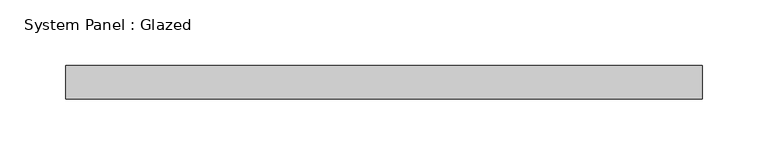
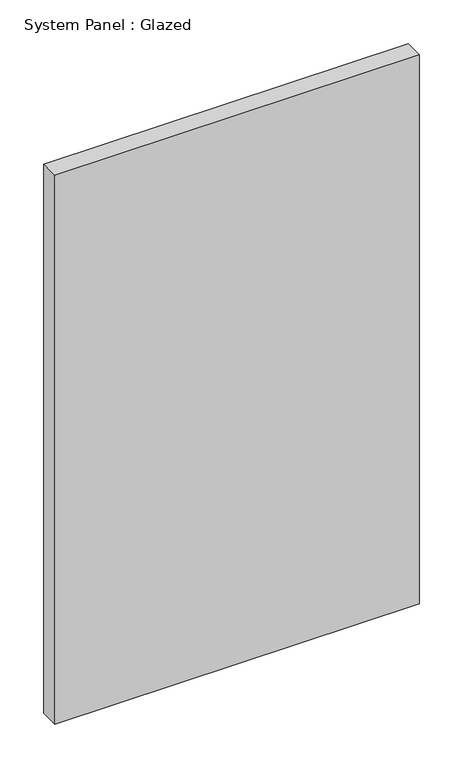
"""IFC4 building model written with IfcOpenShell, lengths in millimetres: plate geometry, System Panel : Glazed."""

from ifc_helpers import new_model, si_unit, origin, origin_with_axes, place, context, project, spatial, polyline, outline, extrude, source, transform, mapped, element, save


def system_panel_glazed_bdd26bb3(model_context):
    return source(origin(), model_context, "Body", "SweptSolid", [
        extrude(outline(polyline([(241.3, 19.05), (-241.3, 19.05), (-241.3, 44.45), (241.3, 44.45), (241.3, 19.05)])), origin_with_axes(), (0.0, 0.0, 1.0), 768.35),
    ])


if __name__ == "__main__":
    model = new_model("IFC4")
    model_context = context("Model", 3, world=origin())
    ifc_project = project(units=[si_unit("LENGTHUNIT", "METRE", prefix="MILLI")], contexts=[model_context])
    site = spatial("IfcSite", under=ifc_project)
    building = spatial("IfcBuilding", under=site)
    placement = place(None, origin())
    system_panel_glazed_shape = system_panel_glazed_bdd26bb3(model_context)
    element("IfcPlate", 1, ObjectType="System Panel : Glazed", at=placement, inside=building, context=model_context, shape_type="MappedRepresentation", body=[
        mapped(system_panel_glazed_shape, transform((0.0, 0.0, 0.0), x_axis=(1.0, 0.0, 0.0), y_axis=(0.0, 1.0, 0.0), z_axis=(0.0, 0.0, 1.0))),
    ])
    save(model, "model.ifc")

# Revit data of these elements
# Type "System Panel : Glazed"
#   Construction Type Id = "GSP4R"
#   Analytic Construction = "1/8 in Pilkington single glazing"
#   Visual Light Transmittance = 0.9
#   Solar Heat Gain Coefficient = 0.86
#   Heat Transfer Coefficient (U) = 1.18115 BTU/(h·ft²·°F)
#   Define Thermal Properties by = 1
# Element 1 (IfcPlate, "System Panel : Glazed")
#   Materials on its faces: "Glass"
# Materials
#   "Glass": class "Glass", colour RGB 0 128 192, transparency 0.75, Description = "Soda Lime Glass", Cost = 0
